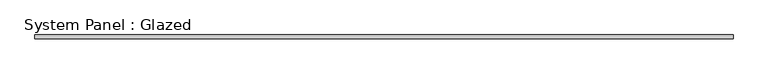
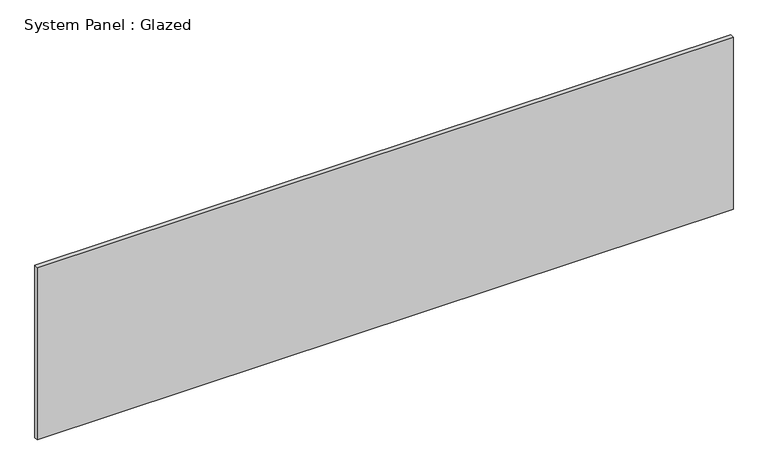
"""IFC4 building model written with IfcOpenShell, lengths in millimetres: plate geometry, System Panel : Glazed."""

from ifc_helpers import new_model, si_unit, origin, origin_with_axes, place, context, project, spatial, polyline, outline, extrude, source, transform, mapped, element, save


def system_panel_glazed_5fd648d4(model_context):
    return source(origin(), model_context, "Body", "SweptSolid", [
        extrude(outline(polyline([(2331.4324687, 19.05), (-2331.4324687, 19.05), (-2331.4324687, 44.45), (2331.4324687, 44.45), (2331.4324687, 19.05)])), origin_with_axes(), (0.0, 0.0, 1.0), 1219.2),
    ])


if __name__ == "__main__":
    model = new_model("IFC4")
    model_context = context("Model", 3, world=origin())
    ifc_project = project(units=[si_unit("LENGTHUNIT", "METRE", prefix="MILLI")], contexts=[model_context])
    site = spatial("IfcSite", under=ifc_project)
    building = spatial("IfcBuilding", under=site)
    placement = place(None, origin())
    system_panel_glazed_shape = system_panel_glazed_5fd648d4(model_context)
    element("IfcPlate", 1, ObjectType="System Panel : Glazed", at=placement, inside=building, context=model_context, shape_type="MappedRepresentation", body=[
        mapped(system_panel_glazed_shape, transform((0.0, 0.0, 0.0), x_axis=(1.0, 0.0, 0.0), y_axis=(0.0, 1.0, 0.0), z_axis=(0.0, 0.0, 1.0))),
    ])
    save(model, "model.ifc")

# Revit data of these elements
# Type "System Panel : Glazed"
#   Construction Type Id = "GSP4R"
#   Analytic Construction = "1/8 in Pilkington single glazing"
#   Visual Light Transmittance = 0.9
#   Solar Heat Gain Coefficient = 0.86
#   Heat Transfer Coefficient (U) = 1.18115 BTU/(h·ft²·°F)
# Element 1 (IfcPlate, "System Panel : Glazed")
#   Materials on its faces: "Glass"
# Materials
#   "Glass": class "Glass", colour RGB 0 128 192, transparency 0.75, Description = "Soda Lime Glass", Cost = 0
